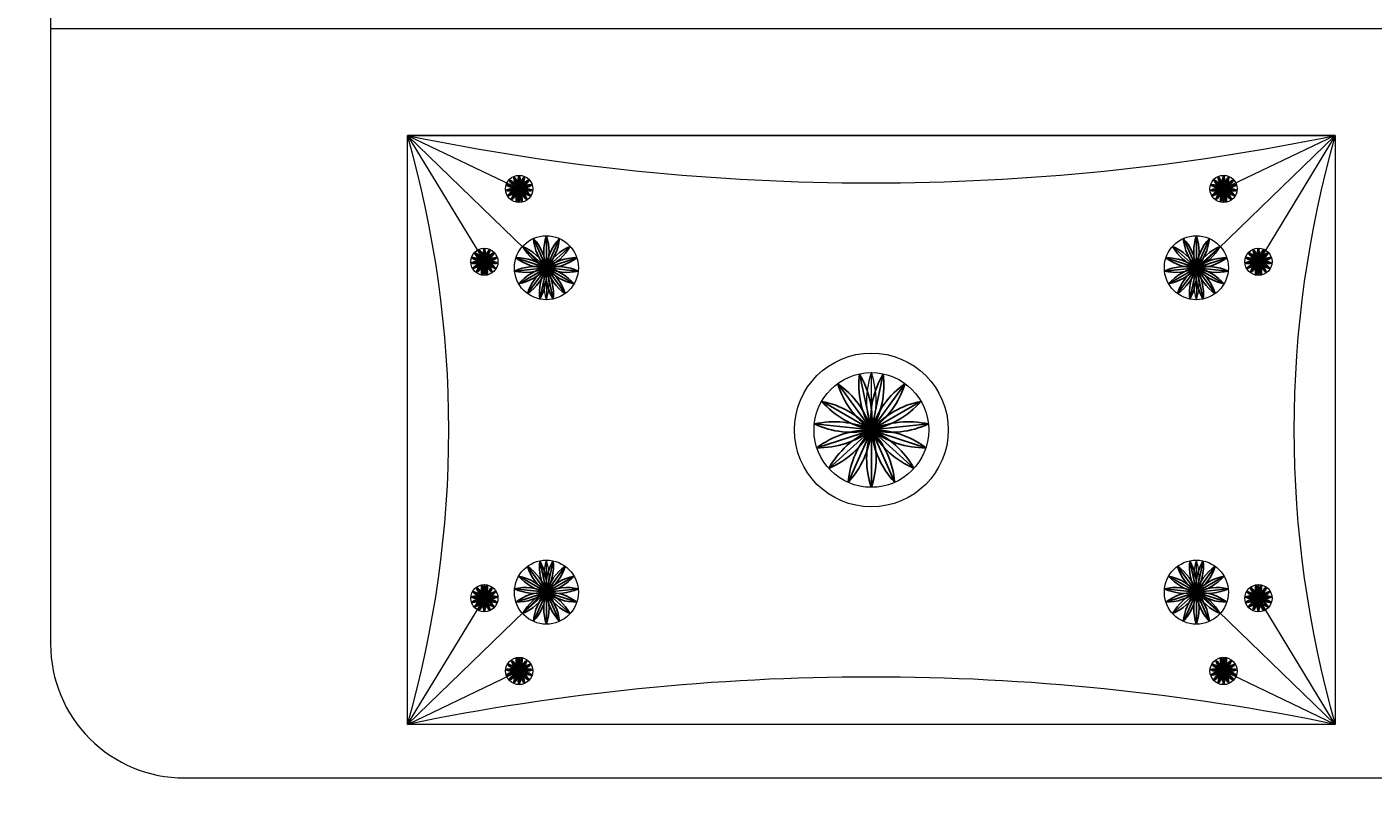
# Model space of a CAD drawing. Units: inches. Extents: x -61 to 1599, y -1316 to 257.
# Tile 47 of 204: x 114 to 149, y -428 to -408. Entities that reach past the tile are written whole.
import ezdxf

# ---------------------------------------------------------------- set-up
doc = ezdxf.new("R2010")
doc.units = ezdxf.units.IN
doc.header["$MEASUREMENT"] = 0
doc.layers.add('A-ANNO-DIMS', color=2, linetype='Continuous', lineweight=18)
doc.layers.add('FURNITURE', color=83, linetype='Continuous', lineweight=18)
doc.layers.add('LT', color=8, linetype='Continuous')
doc.styles.get("Standard").update_dxf_attribs({"font": 'arial.ttf'})
doc.dimstyles.get("Standard").update_dxf_attribs({"dimtxt": 0.18, "dimasz": 0.18, "dimexe": 0.18, "dimexo": 0.0625, "dimgap": 0.09, "dimtad": 0, "dimtih": 1, "dimtoh": 1, "dimdec": 0, "dimzin": 0, "dimdsep": 46, "dimlunit": 3, "dimtxsty": 'Standard', "dimcen": 0.09, "dimadec": 0, "dimazin": 0, "dimtfac": 1, "dimtdec": 0, "dimtofl": 0, "dimtmove": 0, "dimatfit": 3, "dimfxl": 1, "dimtolj": 1, "dimtzin": 0, "dimarcsym": 0})

# ---------------------------------------------------------------- blocks, each defined once
blk = doc.blocks.new('*U15')
at = {"layer": 'LT'}
blk.add_line((0, 0.175), (0, -0.175), dxfattribs=at)
for centre, start, end in [((0.509, 0), 160.9983, 199.0017), ((-0.509, 0), 340.9983, 19.0017)]:
    blk.add_arc(centre, 0.539, start, end, dxfattribs=at)
blk = doc.blocks.new('*U16')
at = {"layer": 'LT', "transparency": 16777216}
for p, rotation in [((-66.642, -18.755), 72), ((-66.605, -18.692), 48.00000000000001), ((-66.546, -18.649), 24), ((-66.404, -18.649), 336.0000000000001), ((-66.345, -18.692), 312), ((-66.308, -18.755), 288.0000000000001), ((-66.649, -18.828), 96), ((-66.627, -18.897), 120), ((-66.578, -18.951), 144), ((-66.512, -18.981), 168.0000000000001), ((-66.439, -18.981), 192), ((-66.372, -18.951), 216), ((-66.323, -18.897), 240), ((-66.301, -18.828), 264)]:
    blk.add_blockref('*U15', p, dxfattribs=dict(at, rotation=rotation))
blk.add_blockref('*U15', (-66.475, -18.634), dxfattribs=at)
blk = doc.blocks.new('*U45')
at = {"layer": 'LT'}
blk.add_line((0, 0.175), (0, -0.175), dxfattribs=at)
for centre, start, end in [((0.509, 0), 160.9983, 199.0017), ((-0.509, 0), 340.9983, 19.0017)]:
    blk.add_arc(centre, 0.539, start, end, dxfattribs=at)
blk = doc.blocks.new('*U46')
at = {"layer": 'LT', "transparency": 16777216}
for p, rotation in [((-66.642, -18.755), 72), ((-66.605, -18.692), 48.00000000000001), ((-66.546, -18.649), 24), ((-66.404, -18.649), 336.0000000000001), ((-66.345, -18.692), 312), ((-66.308, -18.755), 288.0000000000001), ((-66.649, -18.828), 96), ((-66.627, -18.897), 120), ((-66.578, -18.951), 144), ((-66.512, -18.981), 168.0000000000001), ((-66.439, -18.981), 192), ((-66.372, -18.951), 216), ((-66.323, -18.897), 240), ((-66.301, -18.828), 264)]:
    blk.add_blockref('*U45', p, dxfattribs=dict(at, rotation=rotation))
blk.add_blockref('*U45', (-66.475, -18.634), dxfattribs=at)
blk = doc.blocks.new('*U9')
at = {"layer": 'LT'}
blk.add_line((0, 0.175), (0, -0.175), dxfattribs=at)
for centre, start, end in [((0.509, 0), 160.9983, 199.0017), ((-0.509, 0), 340.9983, 19.0017)]:
    blk.add_arc(centre, 0.539, start, end, dxfattribs=at)
blk = doc.blocks.new('*U10')
at = {"layer": 'LT', "transparency": 16777216}
for p, rotation in [((-66.642, -18.755), 72), ((-66.605, -18.692), 48.00000000000001), ((-66.546, -18.649), 24), ((-66.404, -18.649), 336.0000000000001), ((-66.345, -18.692), 312), ((-66.308, -18.755), 288.0000000000001), ((-66.649, -18.828), 96), ((-66.627, -18.897), 120), ((-66.578, -18.951), 144), ((-66.512, -18.981), 168.0000000000001), ((-66.439, -18.981), 192), ((-66.372, -18.951), 216), ((-66.323, -18.897), 240), ((-66.301, -18.828), 264)]:
    blk.add_blockref('*U9', p, dxfattribs=dict(at, rotation=rotation))
blk.add_blockref('*U9', (-66.475, -18.634), dxfattribs=at)
blk = doc.blocks.new('*U39')
at = {"layer": 'LT'}
blk.add_line((0, 0.175), (0, -0.175), dxfattribs=at)
for centre, start, end in [((0.509, 0), 160.9983, 199.0017), ((-0.509, 0), 340.9983, 19.0017)]:
    blk.add_arc(centre, 0.539, start, end, dxfattribs=at)
blk = doc.blocks.new('*U40')
at = {"layer": 'LT', "transparency": 16777216}
for p, rotation in [((-66.642, -18.755), 72), ((-66.605, -18.692), 48.00000000000001), ((-66.546, -18.649), 24), ((-66.404, -18.649), 336.0000000000001), ((-66.345, -18.692), 312), ((-66.308, -18.755), 288.0000000000001), ((-66.649, -18.828), 96), ((-66.627, -18.897), 120), ((-66.578, -18.951), 144), ((-66.512, -18.981), 168.0000000000001), ((-66.439, -18.981), 192), ((-66.372, -18.951), 216), ((-66.323, -18.897), 240), ((-66.301, -18.828), 264)]:
    blk.add_blockref('*U39', p, dxfattribs=dict(at, rotation=rotation))
blk.add_blockref('*U39', (-66.475, -18.634), dxfattribs=at)
blk = doc.blocks.new('*U17')
at = {"layer": 'LT'}
blk.add_line((0, 0.412), (0, -0.412), dxfattribs=at)
for centre, start, end in [((1.198, 0), 160.9983, 199.0017), ((-1.198, 0), 340.9983, 19.0017)]:
    blk.add_arc(centre, 1.267, start, end, dxfattribs=at)
blk = doc.blocks.new('*U18')
at = {"layer": 'LT', "transparency": 16777216}
for p, rotation in [((-156.639, -43.959), 48.00000000000001), ((-156.501, -43.858), 24), ((-156.165, -43.858), 336.0000000000001), ((-156.027, -43.959), 312), ((-156.725, -44.108), 72), ((-155.941, -44.108), 288.0000000000001), ((-156.743, -44.278), 96), ((-156.69, -44.441), 120), ((-156.575, -44.569), 144), ((-156.419, -44.639), 168), ((-156.247, -44.639), 192), ((-156.091, -44.569), 216), ((-155.976, -44.441), 240), ((-155.923, -44.278), 264)]:
    blk.add_blockref('*U17', p, dxfattribs=dict(at, rotation=rotation))
blk.add_blockref('*U17', (-156.333, -43.823), dxfattribs=at)
blk = doc.blocks.new('*U33')
at = {"layer": 'LT'}
blk.add_line((0, 0.412), (0, -0.412), dxfattribs=at)
for centre, start, end in [((1.198, 0), 160.9983, 199.0017), ((-1.198, 0), 340.9983, 19.0017)]:
    blk.add_arc(centre, 1.267, start, end, dxfattribs=at)
blk = doc.blocks.new('*U34')
at = {"layer": 'LT', "transparency": 16777216}
for p, rotation in [((-156.639, -43.959), 48.00000000000001), ((-156.501, -43.858), 24), ((-156.165, -43.858), 336.0000000000001), ((-156.027, -43.959), 312), ((-156.725, -44.108), 72), ((-155.941, -44.108), 288.0000000000001), ((-156.743, -44.278), 96), ((-156.69, -44.441), 120), ((-156.575, -44.569), 144), ((-156.419, -44.639), 168), ((-156.247, -44.639), 192), ((-156.091, -44.569), 216), ((-155.976, -44.441), 240), ((-155.923, -44.278), 264)]:
    blk.add_blockref('*U33', p, dxfattribs=dict(at, rotation=rotation))
blk.add_blockref('*U33', (-156.333, -43.823), dxfattribs=at)
blk = doc.blocks.new('*U11')
at = {"layer": 'LT'}
blk.add_line((0, 0.739), (0, -0.739), dxfattribs=at)
for centre, start, end in [((2.147, 0), 160.9983, 199.0017), ((-2.147, 0), 340.9983, 19.0017)]:
    blk.add_arc(centre, 2.27, start, end, dxfattribs=at)
blk = doc.blocks.new('*U12')
at = {"layer": 'LT', "transparency": 16777216}
for p, rotation in [((-280.542, -78.621), 23.99999999999999), ((-279.941, -78.621), 336.0000000000001), ((-280.791, -78.801), 48.00000000000001), ((-279.692, -78.801), 312), ((-280.945, -79.067), 72), ((-279.539, -79.067), 288.0000000000001), ((-280.977, -79.373), 96), ((-280.882, -79.665), 120), ((-280.676, -79.894), 144), ((-280.395, -80.019), 168), ((-280.088, -80.019), 191.9999999999999), ((-279.807, -79.894), 216), ((-279.602, -79.665), 240), ((-279.507, -79.373), 264)]:
    blk.add_blockref('*U11', p, dxfattribs=dict(at, rotation=rotation))
blk.add_blockref('*U11', (-280.242, -78.557), dxfattribs=at)
blk = doc.blocks.new('*U28')
at = {"layer": 'LT'}
blk.add_line((0, 0.412), (0, -0.412), dxfattribs=at)
for centre, start, end in [((1.198, 0), 160.9983, 199.0017), ((-1.198, 0), 340.9983, 19.0017)]:
    blk.add_arc(centre, 1.267, start, end, dxfattribs=at)
blk = doc.blocks.new('*U44')
at = {"layer": 'LT', "transparency": 16777216}
for p, rotation in [((-156.639, -43.959), 48.00000000000001), ((-156.501, -43.858), 24), ((-156.165, -43.858), 336.0000000000001), ((-156.027, -43.959), 312), ((-156.725, -44.108), 72), ((-155.941, -44.108), 288.0000000000001), ((-156.743, -44.278), 96), ((-156.69, -44.441), 120), ((-156.575, -44.569), 144), ((-156.419, -44.639), 168), ((-156.247, -44.639), 192), ((-156.091, -44.569), 216), ((-155.976, -44.441), 240), ((-155.923, -44.278), 264)]:
    blk.add_blockref('*U28', p, dxfattribs=dict(at, rotation=rotation))
blk.add_blockref('*U28', (-156.333, -43.823), dxfattribs=at)
blk = doc.blocks.new('*U13')
at = {"layer": 'LT'}
blk.add_line((0, 0.412), (0, -0.412), dxfattribs=at)
for centre, start, end in [((1.198, 0), 160.9983, 199.0017), ((-1.198, 0), 340.9983, 19.0017)]:
    blk.add_arc(centre, 1.267, start, end, dxfattribs=at)
blk = doc.blocks.new('*U14')
at = {"layer": 'LT', "transparency": 16777216}
for p, rotation in [((-156.639, -43.959), 48.00000000000001), ((-156.501, -43.858), 24), ((-156.165, -43.858), 336.0000000000001), ((-156.027, -43.959), 312), ((-156.725, -44.108), 72), ((-155.941, -44.108), 288.0000000000001), ((-156.743, -44.278), 96), ((-156.69, -44.441), 120), ((-156.575, -44.569), 144), ((-156.419, -44.639), 168), ((-156.247, -44.639), 192), ((-156.091, -44.569), 216), ((-155.976, -44.441), 240), ((-155.923, -44.278), 264)]:
    blk.add_blockref('*U13', p, dxfattribs=dict(at, rotation=rotation))
blk.add_blockref('*U13', (-156.333, -43.823), dxfattribs=at)
blk = doc.blocks.new('*U19')
at = {"layer": 'LT'}
blk.add_line((0, 0.175), (0, -0.175), dxfattribs=at)
for centre, start, end in [((0.509, 0), 160.9983, 199.0017), ((-0.509, 0), 340.9983, 19.0017)]:
    blk.add_arc(centre, 0.539, start, end, dxfattribs=at)
blk = doc.blocks.new('*U6')
at = {"layer": 'LT', "transparency": 16777216}
for p, rotation in [((-66.642, -18.755), 72), ((-66.605, -18.692), 48.00000000000001), ((-66.546, -18.649), 24), ((-66.404, -18.649), 336.0000000000001), ((-66.345, -18.692), 312), ((-66.308, -18.755), 288.0000000000001), ((-66.649, -18.828), 96), ((-66.627, -18.897), 120), ((-66.578, -18.951), 144), ((-66.512, -18.981), 168.0000000000001), ((-66.439, -18.981), 192), ((-66.372, -18.951), 216), ((-66.323, -18.897), 240), ((-66.301, -18.828), 264)]:
    blk.add_blockref('*U19', p, dxfattribs=dict(at, rotation=rotation))
blk.add_blockref('*U19', (-66.475, -18.634), dxfattribs=at)
blk = doc.blocks.new('*U35')
at = {"layer": 'LT'}
blk.add_line((0, 0.175), (0, -0.175), dxfattribs=at)
for centre, start, end in [((0.509, 0), 160.9983, 199.0017), ((-0.509, 0), 340.9983, 19.0017)]:
    blk.add_arc(centre, 0.539, start, end, dxfattribs=at)
blk = doc.blocks.new('*U36')
at = {"layer": 'LT', "transparency": 16777216}
for p, rotation in [((-66.642, -18.755), 72), ((-66.605, -18.692), 48.00000000000001), ((-66.546, -18.649), 24), ((-66.404, -18.649), 336.0000000000001), ((-66.345, -18.692), 312), ((-66.308, -18.755), 288.0000000000001), ((-66.649, -18.828), 96), ((-66.627, -18.897), 120), ((-66.578, -18.951), 144), ((-66.512, -18.981), 168.0000000000001), ((-66.439, -18.981), 192), ((-66.372, -18.951), 216), ((-66.323, -18.897), 240), ((-66.301, -18.828), 264)]:
    blk.add_blockref('*U35', p, dxfattribs=dict(at, rotation=rotation))
blk.add_blockref('*U35', (-66.475, -18.634), dxfattribs=at)
blk = doc.blocks.new('*U7')
at = {"layer": 'LT'}
blk.add_line((0, 0.175), (0, -0.175), dxfattribs=at)
for centre, start, end in [((0.509, 0), 160.9983, 199.0017), ((-0.509, 0), 340.9983, 19.0017)]:
    blk.add_arc(centre, 0.539, start, end, dxfattribs=at)
blk = doc.blocks.new('*U8')
at = {"layer": 'LT', "transparency": 16777216}
for p, rotation in [((-66.642, -18.755), 72), ((-66.605, -18.692), 48.00000000000001), ((-66.546, -18.649), 24), ((-66.404, -18.649), 336.0000000000001), ((-66.345, -18.692), 312), ((-66.308, -18.755), 288.0000000000001), ((-66.649, -18.828), 96), ((-66.627, -18.897), 120), ((-66.578, -18.951), 144), ((-66.512, -18.981), 168.0000000000001), ((-66.439, -18.981), 192), ((-66.372, -18.951), 216), ((-66.323, -18.897), 240), ((-66.301, -18.828), 264)]:
    blk.add_blockref('*U7', p, dxfattribs=dict(at, rotation=rotation))
blk.add_blockref('*U7', (-66.475, -18.634), dxfattribs=at)
blk = doc.blocks.new('*U37')
at = {"layer": 'LT'}
blk.add_line((0, 0.175), (0, -0.175), dxfattribs=at)
for centre, start, end in [((0.509, 0), 160.9983, 199.0017), ((-0.509, 0), 340.9983, 19.0017)]:
    blk.add_arc(centre, 0.539, start, end, dxfattribs=at)
blk = doc.blocks.new('*U38')
at = {"layer": 'LT', "transparency": 16777216}
for p, rotation in [((-66.642, -18.755), 72), ((-66.605, -18.692), 48.00000000000001), ((-66.546, -18.649), 24), ((-66.404, -18.649), 336.0000000000001), ((-66.345, -18.692), 312), ((-66.308, -18.755), 288.0000000000001), ((-66.649, -18.828), 96), ((-66.627, -18.897), 120), ((-66.578, -18.951), 144), ((-66.512, -18.981), 168.0000000000001), ((-66.439, -18.981), 192), ((-66.372, -18.951), 216), ((-66.323, -18.897), 240), ((-66.301, -18.828), 264)]:
    blk.add_blockref('*U37', p, dxfattribs=dict(at, rotation=rotation))
blk.add_blockref('*U37', (-66.475, -18.634), dxfattribs=at)
blk = doc.blocks.new('BED-DOUBLE')
for p, q in [((1.272, 19.317), (70.263, 19.317)), ((10.471, 1.379), (10.471, 16.557)), ((34.388, 16.557), (10.471, 16.557)), ((10.471, 16.557), (13.35, 15.18)), ((10.471, 16.557), (14.039, 13.107)), ((10.471, 16.557), (12.454, 13.305)), ((34.388, 16.557), (30.82, 13.107)), ((34.388, 16.557), (31.508, 15.18)), ((34.388, 16.557), (32.405, 13.305)), ((13.35, 15.18), (13.35, 14.829)), ((31.508, 15.18), (31.508, 14.829)), ((12.454, 13.305), (12.454, 12.955)), ((32.405, 13.305), (32.405, 12.955)), ((14.052, 13.149), (14.052, 12.324)), ((30.806, 13.149), (30.806, 12.324)), ((22.429, 8.968), (22.429, 10.447)), ((14.052, 4.788), (14.052, 5.613)), ((30.806, 4.788), (30.806, 5.613)), ((12.454, 4.631), (12.454, 4.982)), ((32.405, 4.631), (32.405, 4.982)), ((10.471, 1.379), (14.039, 4.83)), ((10.471, 1.379), (12.454, 4.631)), ((34.388, 1.379), (30.82, 4.83)), ((34.388, 1.379), (32.405, 4.631)), ((13.35, 2.756), (13.35, 3.107)), ((31.508, 2.756), (31.508, 3.107)), ((10.471, 1.379), (13.35, 2.756)), ((34.388, 1.379), (31.508, 2.756)), ((34.388, 1.379), (34.388, 1.379))]:
    blk.add_line(p, q)
for points in [[(1.272, 88.537), (1.272, 3.449, 0.414214), (4.722, 0), (66.813, 0, 0.414214), (70.263, 3.449), (70.263, 88.537, 0.414214), (66.813, 91.987), (4.722, 91.987, 0.414214)], [(13.35, 15.18, 0.167358), (13.35, 14.829, 0.167358)], [(12.454, 13.305, 0.167358), (12.454, 12.955, 0.167358)], [(32.405, 12.955, 0.167358), (32.405, 13.305, 0.167358)], [(14.052, 13.149, 0.167358), (14.052, 12.324, 0.167358)], [(30.806, 12.324, 0.167358), (30.806, 13.149, 0.167358)], [(22.429, 8.968, 0.167358), (22.429, 10.447, 0.167358)], [(14.052, 5.613, 0.167358), (14.052, 4.788, 0.167358)], [(30.806, 4.788, 0.167358), (30.806, 5.613, 0.167358)], [(12.454, 4.982, 0.167358), (12.454, 4.631, 0.167358)], [(32.405, 4.631, 0.167358), (32.405, 4.982, 0.167358)], [(13.35, 3.107, 0.167358), (13.35, 2.756, 0.167358)], [(31.508, 2.756, 0.167358), (31.508, 3.107, 0.167358)]]:
    blk.add_lwpolyline(points, format="xyb", close=True)
blk.add_lwpolyline([(34.388, 16.557), (34.388, 1.379), (10.471, 1.379), (10.471, 16.557), (34.388, 16.557), (34.388, 1.379), (10.471, 1.379)])
for centre, radius in [((13.35, 15.18), 0.351), ((31.508, 15.18), 0.351), ((14.052, 13.149), 0.825), ((30.806, 13.149), 0.825), ((12.454, 13.305), 0.351), ((32.405, 13.305), 0.351), ((22.429, 8.968), 1.982), ((22.429, 8.968), 1.478), ((14.052, 4.788), 0.825), ((30.806, 4.788), 0.825), ((12.454, 4.631), 0.351), ((32.405, 4.631), 0.351), ((13.35, 2.756), 0.351), ((31.508, 2.756), 0.351)]:
    blk.add_circle(centre, radius)
for centre, radius, start, end in [((-16.003, 8.968), 27.54, 344.0046, 15.9954), ((22.429, 74.54), 59.203, 258.34678, 281.65322), ((60.861, 8.968), 27.54, 164.0046, 195.9954), ((32.017, 15.005), 0.539, 160.9983, 199.0017), ((30.999, 15.005), 0.539, 340.9983, 19.0017), ((22.429, -56.603), 59.203, 78.34678, 101.65322)]:
    blk.add_arc(centre, radius, start, end)
for name, p in [('*U40', (79.825, 33.99)), ('*U34', (170.385, 57.384)), ('*U46', (78.929, 32.115))]:
    blk.add_blockref(name, p)
at = {"extrusion": (0, 0, -1), "zscale": -1}
for name, p in [('*U36', (34.967, 33.99)), ('*U14', (125.527, 57.384)), ('*U38', (34.07, 32.115))]:
    blk.add_blockref(name, p, dxfattribs=at)
at = {"rotation": 180}
for name, p in [('*U12', (-257.812, -70.328)), ('*U44', (-125.527, -39.447)), ('*U8', (-34.07, -14.178)), ('*U6', (-34.967, -16.053))]:
    blk.add_blockref(name, p, dxfattribs=at)
at = {"extrusion": (0, 0, -1), "zscale": -1, "rotation": 180}
for name, p in [('*U18', (-170.385, -39.447)), ('*U16', (-78.929, -14.178)), ('*U10', (-79.825, -16.053))]:
    blk.add_blockref(name, p, dxfattribs=at)
blk = doc.blocks.new('*D687')
at = {"layer": 'A-ANNO-DIMS', "color": 0, "lineweight": -2, "transparency": 16777216}
for p, q in [((289.418, 181.677), (-61.077, 181.677)), ((-60.897, 181.497), (-60.897, -528.952)), ((-60.897, -1239.765), (-60.897, -529.316)), ((319.64, -1239.945), (-61.077, -1239.945))]:
    blk.add_line(p, q, dxfattribs=at)
at = {"layer": 'A-ANNO-DIMS', "color": 0, "transparency": 16777216}
for points in [[(-60.927, 181.497), (-60.867, 181.497), (-60.897, 181.677)], [(-60.927, -1239.765), (-60.867, -1239.765), (-60.897, -1239.945)]]:
    blk.add_solid(points, dxfattribs=at)
at = {"layer": 'DEFPOINTS', "color": 0, "transparency": 16777216}
for p in [(289.481, 181.677), (-60.897, -1239.945), (319.703, -1239.945)]:
    blk.add_point(p, dxfattribs=at)
at = {"layer": 'A-ANNO-DIMS', "color": 0, "transparency": 16777216, "insert": (-60.897, -529.134), "char_height": 0.18, "attachment_point": 5}
blk.add_mtext('\\A1;1421.6', dxfattribs=at)
blk = doc.blocks.new('*D699')
at = {"layer": 'A-ANNO-DIMS', "color": 0, "lineweight": -2, "transparency": 16777216}
for p, q in [((835.64, -167.169), (-61.077, -167.169)), ((-60.897, -167.349), (-60.897, -306.726)), ((-60.897, -446.466), (-60.897, -307.09)), ((841.64, -446.646), (-61.077, -446.646))]:
    blk.add_line(p, q, dxfattribs=at)
at = {"layer": 'A-ANNO-DIMS', "color": 0, "transparency": 16777216}
for points in [[(-60.927, -167.349), (-60.867, -167.349), (-60.897, -167.169)], [(-60.927, -446.466), (-60.867, -446.466), (-60.897, -446.646)]]:
    blk.add_solid(points, dxfattribs=at)
at = {"layer": 'DEFPOINTS', "color": 0, "transparency": 16777216}
for p in [(835.703, -167.169), (-60.897, -446.646), (841.703, -446.646)]:
    blk.add_point(p, dxfattribs=at)
at = {"layer": 'A-ANNO-DIMS', "color": 0, "transparency": 16777216, "insert": (-60.897, -306.908), "char_height": 0.18, "attachment_point": 5}
blk.add_mtext('\\A1;279.5', dxfattribs=at)
blk = doc.blocks.new('*D700')
at = {"layer": 'A-ANNO-DIMS', "color": 0, "lineweight": -2, "transparency": 16777216}
for p, q in [((14.703, -616.882), (14.703, 257.457)), ((14.883, 257.277), (96.772, 257.277)), ((179.572, 257.277), (97.683, 257.277)), ((179.752, -616.882), (179.752, 257.457))]:
    blk.add_line(p, q, dxfattribs=at)
at = {"layer": 'A-ANNO-DIMS', "color": 0, "transparency": 16777216}
for points in [[(14.883, 257.307), (14.883, 257.247), (14.703, 257.277)], [(179.572, 257.307), (179.572, 257.247), (179.752, 257.277)]]:
    blk.add_solid(points, dxfattribs=at)
at = {"layer": 'DEFPOINTS', "color": 0, "transparency": 16777216}
for p in [(179.752, 257.277), (14.703, -616.945), (179.752, -616.945)]:
    blk.add_point(p, dxfattribs=at)
at = {"layer": 'A-ANNO-DIMS', "color": 0, "transparency": 16777216, "insert": (97.227, 257.277), "char_height": 0.18, "attachment_point": 5}
blk.add_mtext('\\A1;165.05', dxfattribs=at)

msp = doc.modelspace()

# ---------------------------------------------------------------- block references
at = {"layer": 'FURNITURE'}
msp.add_blockref('BED-DOUBLE', (113.2612, -427.6961), dxfattribs=at)

# ---------------------------------------------------------------- dimensions: what is measured, and where the dimension line sits
at = {"layer": 'A-ANNO-DIMS'}
dim = msp.add_linear_dim(base=(179.7521, 257.2771), p1=(14.7028, -616.9446), p2=(179.7521, -616.9446), dimstyle='Standard', override={"dimdec": 2, "dimlfac": 1, "dimrnd": 0, "dimzin": 0, "dimdsep": 46, "dimlunit": 2}, dxfattribs=at)
dim.commit()
dim.dimension.update_dxf_attribs({"geometry": '*D700', "text_midpoint": (97.2274, 257.2771)})
for base, p1, p2, picture, middle in [((-60.8972, -1239.9446), (289.4807, 181.6771), (319.7028, -1239.9446), '*D687', (-60.8972, -529.1337)), ((-60.8972, -446.6462), (835.7028, -167.169), (841.7028, -446.6462), '*D699', (-60.8972, -306.9076))]:
    dim = msp.add_linear_dim(base=base, p1=p1, p2=p2, angle=90, dimstyle='Standard', override={"dimdec": 1, "dimlfac": 1, "dimrnd": 0, "dimzin": 0, "dimdsep": 46, "dimlunit": 2}, dxfattribs=at)
    dim.commit()
    dim.dimension.update_dxf_attribs({"geometry": picture, "text_midpoint": middle})

doc.saveas('drawing.dxf')
